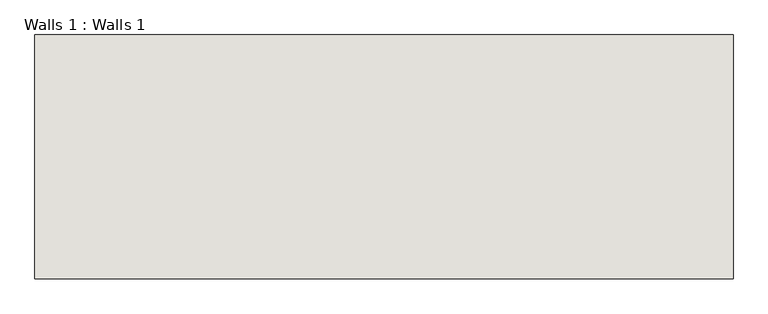
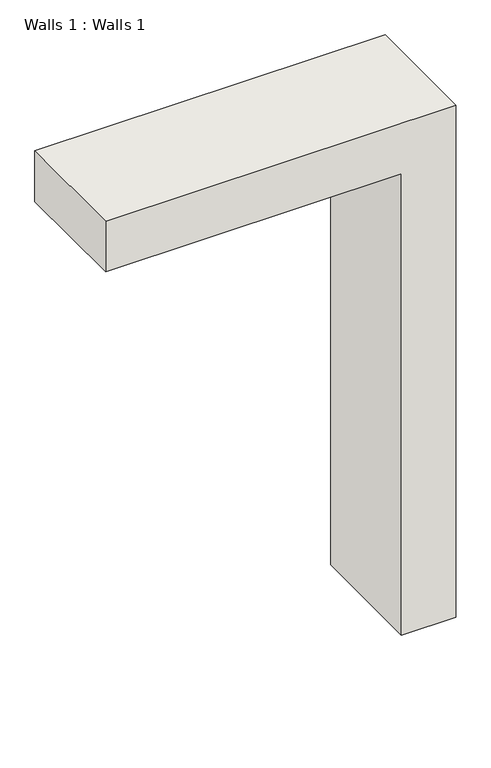
"""IFC4 building model written with IfcOpenShell, lengths in millimetres: wall geometry, Walls 1 : Walls 1."""

from ifc_helpers import new_model, si_unit, frame, origin, place, context, project, spatial, polyline, outline, extrude, source, transform, mapped, element, save


def walls_1_walls_1_8bdf3cb7(model_context):
    return source(origin(), model_context, "Body", "SweptSolid", [
        extrude(outline(polyline([(2762.6009455, -14377.0117787), (2762.6009455, -16165.0135961), (2489.2, -16165.0135961), (2489.2, -14655.4242152), (0.0, -14655.4242152), (0.0, -14377.0117787), (2762.6009455, -14377.0117787)])), frame((0.0, -4015.5522803, 0.0), z_axis=(0.0, 1.0, 0.0), x_axis=(0.0, 0.0, 1.0)), (0.0, 0.0, 1.0), 624.6341905),
    ])


if __name__ == "__main__":
    model = new_model("IFC4")
    model_context = context("Model", 3, world=origin())
    ifc_project = project(units=[si_unit("LENGTHUNIT", "METRE", prefix="MILLI")], contexts=[model_context])
    site = spatial("IfcSite", under=ifc_project)
    building = spatial("IfcBuilding", under=site)
    placement = place(None, origin())
    walls_1_walls_1_shape = walls_1_walls_1_8bdf3cb7(model_context)
    element("IfcWall", 1, ObjectType="Walls 1 : Walls 1", at=placement, inside=building, context=model_context, shape_type="MappedRepresentation", body=[
        mapped(walls_1_walls_1_shape, transform((0.0, 0.0, 0.0), x_axis=(1.0, 0.0, 0.0), y_axis=(0.0, 1.0, 0.0), z_axis=(0.0, 0.0, 1.0))),
    ])
    save(model, "model.ifc")

# Revit data of these elements
# Element 1 (IfcWall, "Walls 1 : Walls 1")
#   Materials on its faces: "Default Wall"
# Materials
#   "Default Wall": colour RGB 80 80 80, transparency 0
